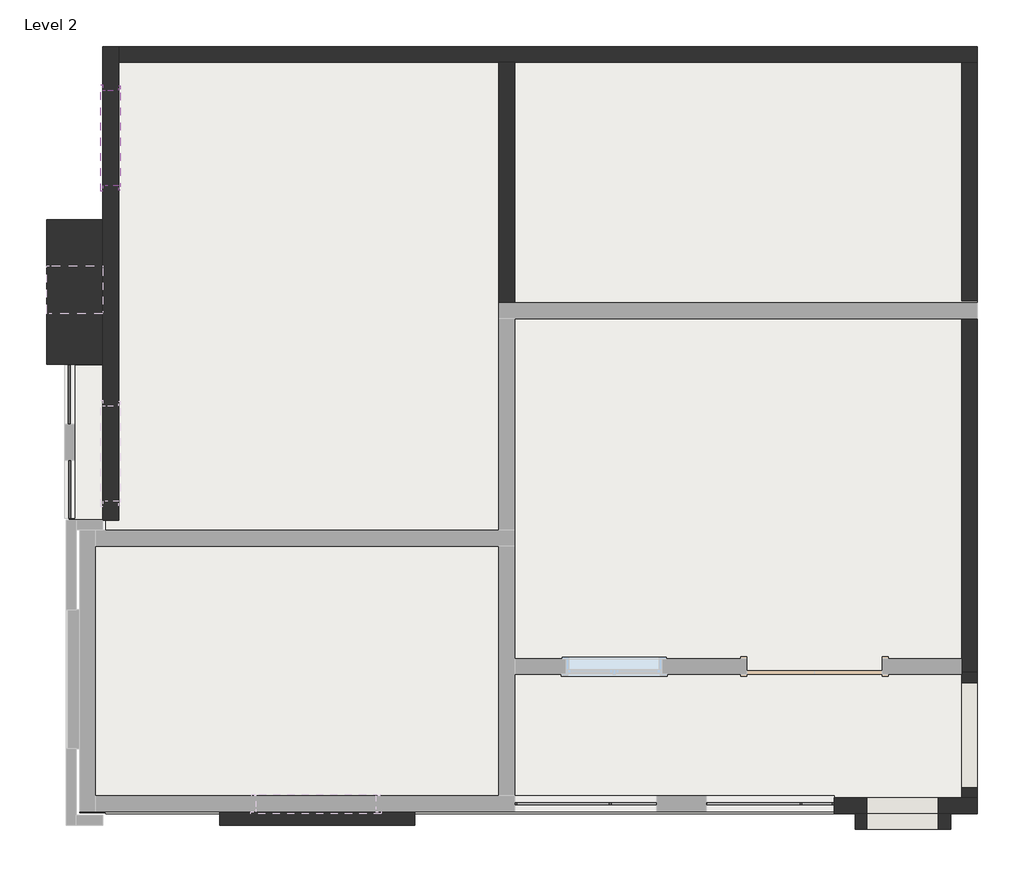
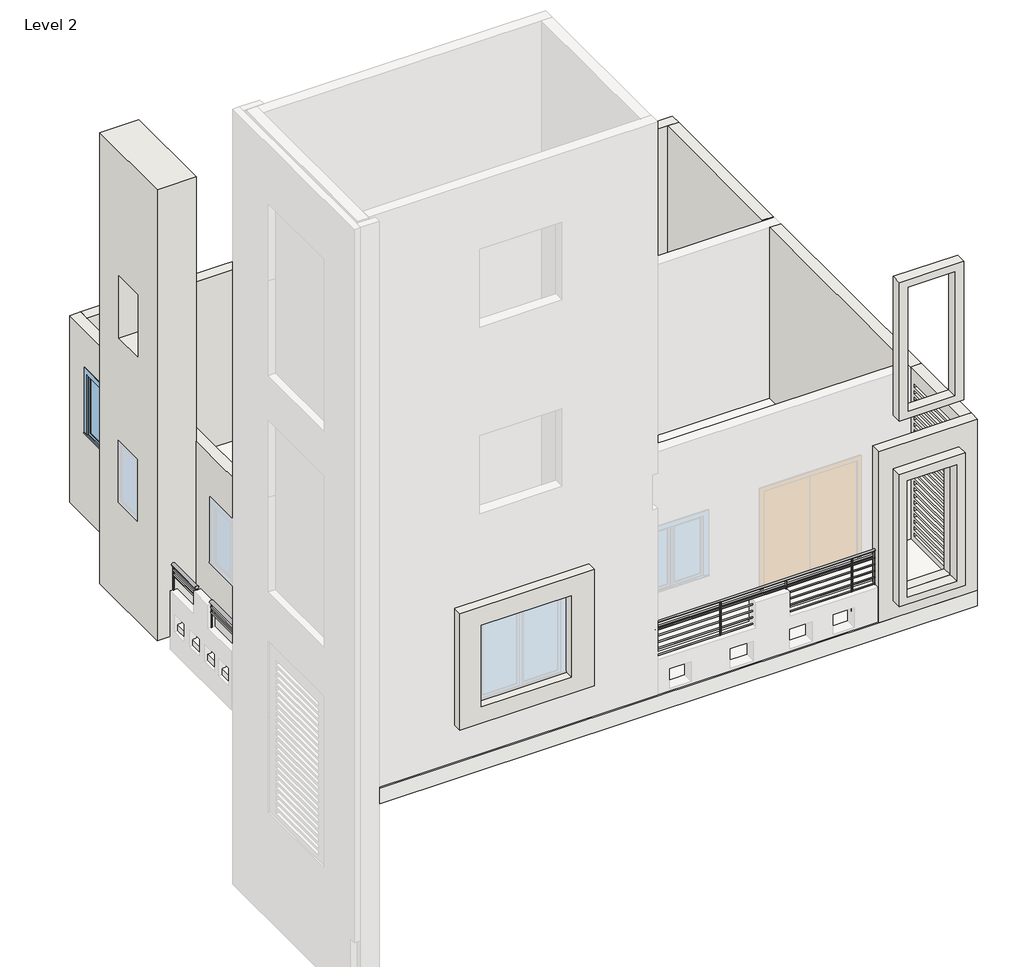
# One storey, part 2 of 2: 10 walls, 3 railings, 1 roof, 1 window.
"""IFC4 building model written with IfcOpenShell, lengths in millimetres."""

from ifc_helpers import new_model, si_unit, point, frame, frame_2d, origin, place, context, project, spatial, polyline, circle_curve, ellipse_curve, trimmed, segment, composite_curve, outline, extrude, faceted_brep, transform, mapped, element, save
from ifc_brep_helpers import plane_surface, extruded_surface, advanced_brep
from components import walls_1_walls_1_b1444295, walls_4_walls_4_8c60a96c, walls_5_walls_5_33b50d55, window_0862ab64

model = new_model("IFC4")

# Units and contexts
model_context = context("Model", 3, world=origin())
ifc_project = project(units=[si_unit("LENGTHUNIT", "METRE", prefix="MILLI")], contexts=[model_context])

# Site, building, storey
site = spatial("IfcSite", under=ifc_project)
building = spatial("IfcBuilding", under=site)
storey = spatial("IfcBuildingStorey", under=building, Name="Level 2", Elevation=3657.6)

# Railings
placement = place(None, origin())
element("IfcRailing", 1, ObjectType="Glass Panel - Bottom Fill", at=placement, inside=storey, context=model_context, shape_type="SolidModel", body=[
    advanced_brep(
    [(-10443.9247472, 7286.192958, 5059.6601563), (-10520.1247472, 7286.192958, 5059.6601563), (-10443.9247472, 6531.4144874, 5059.6601563), (-10520.1247472, 6531.4144874, 5059.6601563)],
    [
        (0, 1, ellipse_curve(frame((-10482.0247472, 7286.192958, 5059.6601563), z_axis=(0.0, 1.0, 0.0), x_axis=(-1.0, 0.0, 0.0)), 38.1, 28.575)),
        (1, 0, ellipse_curve(frame((-10482.0247472, 7286.192958, 5059.6601563), z_axis=(0.0, 1.0, 0.0), x_axis=(-1.0, 0.0, 0.0)), 38.1, 28.575)),
        (2, 3, ellipse_curve(frame((-10482.0247472, 6531.4144874, 5059.6601563), z_axis=(0.0, -1.0, 0.0), x_axis=(-1.0, 0.0, 0.0)), 38.1, 28.575)),
        (3, 2, ellipse_curve(frame((-10482.0247472, 6531.4144874, 5059.6601563), z_axis=(0.0, -1.0, 0.0), x_axis=(-1.0, 0.0, 0.0)), 38.1, 28.575)),
        (0, 2),
        (3, 1),
    ],
    [
        plane_surface(frame((-10482.0247472, 7286.192958, 5059.6601563), z_axis=(0.0, 1.0, 0.0), x_axis=(0.0, 0.0, -1.0))),
        plane_surface(frame((-10482.0247472, 6531.4144874, 5059.6601563), z_axis=(0.0, -1.0, 0.0), x_axis=(0.0, 0.0, -1.0))),
        extruded_surface(trimmed(ellipse_curve(frame((-10482.0247472, 6531.4144874, 5059.6601563), z_axis=(0.0, 1.0, 0.0), x_axis=(-1.0, 0.0, 0.0)), 38.1, 28.575), [point((-10443.9247472, 6531.4144874, 5059.6601563))], [point((-10520.1247472, 6531.4144874, 5059.6601563))], True, "CARTESIAN"), (0.0, 754.7784705999993, 0.0), 754.7784705999993),
        extruded_surface(trimmed(ellipse_curve(frame((-10482.0247472, 6531.4144874, 5059.6601563), z_axis=(0.0, 1.0, 0.0), x_axis=(-1.0, 0.0, 0.0)), 38.1, 28.575), [point((-10520.1247472, 6531.4144874, 5059.6601563))], [point((-10443.9247472, 6531.4144874, 5059.6601563))], True, "CARTESIAN"), (0.0, 754.7784705999993, 0.0), 754.7784705999993),
    ],
    [
        (0, [[1, 2]]),
        (1, [[3, 4]]),
        (2, [[-1, 5, -4, 6]]),
        (3, [[-2, -6, -3, -5]]),
    ],
),
    extrude(outline(polyline([(-10494.7247472, 7286.192958), (-10469.3247472, 7286.192958), (-10469.3247472, 6531.4144874), (-10494.7247472, 6531.4144874), (-10494.7247472, 7286.192958)])), frame((0.0, 0.0, 4945.3601562), z_axis=(0.0, 0.0, 1.0), x_axis=(1.0, 0.0, 0.0)), (0.0, 0.0, 1.0), 25.4),
    extrude(outline(polyline([(-10494.7247472, 7286.192958), (-10469.3247472, 7286.192958), (-10469.3247472, 6531.4144874), (-10494.7247472, 6531.4144874), (-10494.7247472, 7286.192958)])), frame((0.0, 0.0, 4843.7601563), z_axis=(0.0, 0.0, 1.0), x_axis=(1.0, 0.0, 0.0)), (0.0, 0.0, 1.0), 25.4),
    extrude(outline(polyline([(-10491.5497472, 6544.1144874), (-10472.4997472, 6544.1144874), (-10472.4997472, 6525.0644874), (-10491.5497472, 6525.0644874), (-10491.5497472, 6544.1144874)])), frame((0.0, 0.0, 4145.2601563), z_axis=(0.0, 0.0, 1.0), x_axis=(1.0, 0.0, 0.0)), (0.0, 0.0, 1.0), 885.6788223),
    extrude(outline(polyline([(-10491.5497472, 7292.542958), (-10472.4997472, 7292.542958), (-10472.4997472, 7273.492958), (-10491.5497472, 7273.492958), (-10491.5497472, 7292.542958)])), frame((0.0, 0.0, 4145.2601563), z_axis=(0.0, 0.0, 1.0), x_axis=(1.0, 0.0, 0.0)), (0.0, 0.0, 1.0), 885.6788223),
])
element("IfcRailing", 2, ObjectType="Glass Panel - Bottom Fill", at=placement, inside=storey, context=model_context, shape_type="SolidModel", body=[
    advanced_brep(
    [(-10437.5747472, 6074.2144874, 5059.6601563), (-10513.7747472, 6074.2144874, 5059.6601563), (-10437.5747472, 5330.392958, 5059.6601563), (-10513.7747472, 5330.392958, 5059.6601563)],
    [
        (0, 1, ellipse_curve(frame((-10475.6747472, 6074.2144874, 5059.6601563), z_axis=(0.0, 1.0, 0.0), x_axis=(-1.0, 0.0, 0.0)), 38.1, 28.575)),
        (1, 0, ellipse_curve(frame((-10475.6747472, 6074.2144874, 5059.6601563), z_axis=(0.0, 1.0, 0.0), x_axis=(-1.0, 0.0, 0.0)), 38.1, 28.575)),
        (2, 3, ellipse_curve(frame((-10475.6747472, 5330.392958, 5059.6601563), z_axis=(0.0, -1.0, 0.0), x_axis=(-1.0, 0.0, 0.0)), 38.1, 28.575)),
        (3, 2, ellipse_curve(frame((-10475.6747472, 5330.392958, 5059.6601563), z_axis=(0.0, -1.0, 0.0), x_axis=(-1.0, 0.0, 0.0)), 38.1, 28.575)),
        (0, 2),
        (3, 1),
    ],
    [
        plane_surface(frame((-10475.6747472, 6074.2144874, 5059.6601563), z_axis=(0.0, 1.0, 0.0), x_axis=(0.0, 0.0, -1.0))),
        plane_surface(frame((-10475.6747472, 5330.392958, 5059.6601563), z_axis=(0.0, -1.0, 0.0), x_axis=(0.0, 0.0, -1.0))),
        extruded_surface(trimmed(ellipse_curve(frame((-10475.6747472, 5330.392958, 5059.6601563), z_axis=(0.0, 1.0, 0.0), x_axis=(-1.0, 0.0, 0.0)), 38.1, 28.575), [point((-10437.5747472, 5330.392958, 5059.6601563))], [point((-10513.7747472, 5330.392958, 5059.6601563))], True, "CARTESIAN"), (0.0, 743.8215293999992, 0.0), 743.8215293999992),
        extruded_surface(trimmed(ellipse_curve(frame((-10475.6747472, 5330.392958, 5059.6601563), z_axis=(0.0, 1.0, 0.0), x_axis=(-1.0, 0.0, 0.0)), 38.1, 28.575), [point((-10513.7747472, 5330.392958, 5059.6601563))], [point((-10437.5747472, 5330.392958, 5059.6601563))], True, "CARTESIAN"), (0.0, 743.8215293999992, 0.0), 743.8215293999992),
    ],
    [
        (0, [[1, 2]]),
        (1, [[3, 4]]),
        (2, [[-1, 5, -4, 6]]),
        (3, [[-2, -6, -3, -5]]),
    ],
),
    extrude(outline(polyline([(-10488.3747472, 6074.2144874), (-10462.9747472, 6074.2144874), (-10462.9747472, 5330.392958), (-10488.3747472, 5330.392958), (-10488.3747472, 6074.2144874)])), frame((0.0, 0.0, 4945.3601562), z_axis=(0.0, 0.0, 1.0), x_axis=(1.0, 0.0, 0.0)), (0.0, 0.0, 1.0), 25.4),
    extrude(outline(polyline([(-10488.3747472, 6074.2144874), (-10462.9747472, 6074.2144874), (-10462.9747472, 5330.392958), (-10488.3747472, 5330.392958), (-10488.3747472, 6074.2144874)])), frame((0.0, 0.0, 4843.7601563), z_axis=(0.0, 0.0, 1.0), x_axis=(1.0, 0.0, 0.0)), (0.0, 0.0, 1.0), 25.4),
    extrude(outline(polyline([(-10485.1997472, 5343.092958), (-10466.1497472, 5343.092958), (-10466.1497472, 5324.042958), (-10485.1997472, 5324.042958), (-10485.1997472, 5343.092958)])), frame((0.0, 0.0, 4145.2601563), z_axis=(0.0, 0.0, 1.0), x_axis=(1.0, 0.0, 0.0)), (0.0, 0.0, 1.0), 885.6788223),
    extrude(outline(polyline([(-10485.1997472, 6080.5644874), (-10466.1497472, 6080.5644874), (-10466.1497472, 6061.5144874), (-10485.1997472, 6061.5144874), (-10485.1997472, 6080.5644874)])), frame((0.0, 0.0, 4145.2601563), z_axis=(0.0, 0.0, 1.0), x_axis=(1.0, 0.0, 0.0)), (0.0, 0.0, 1.0), 885.6788223),
])
element("IfcRailing", 3, ObjectType="Guardrail - Pipe", at=placement, inside=storey, context=model_context, shape_type="SweptSolid", body=[
    extrude(outline(composite_curve([segment(trimmed(circle_curve(frame_2d((1758.4484482, 5162.55)), 19.05), [point((1739.3984482, 5162.55))], [point((1777.4984482, 5162.55))], False, "CARTESIAN"), True, "CONTINUOUS"), segment(trimmed(circle_curve(frame_2d((1758.4484482, 5162.55)), 19.05), [point((1777.4984482, 5162.55))], [point((1739.3984482, 5162.55))], False, "CARTESIAN"), True, "CONTINUOUS")], self_intersect=False)), frame((-4789.9857575, 0.0, 0.0), z_axis=(1.0, 0.0, 0.0), x_axis=(0.0, 1.0, 0.0)), (0.0, 0.0, 1.0), 4083.7860103),
    extrude(outline(composite_curve([segment(trimmed(circle_curve(frame_2d((1682.2484482, 5314.95)), 19.05), [point((1663.1984482, 5314.95))], [point((1701.2984482, 5314.95))], False, "CARTESIAN"), True, "CONTINUOUS"), segment(trimmed(circle_curve(frame_2d((1682.2484482, 5314.95)), 19.05), [point((1701.2984482, 5314.95))], [point((1663.1984482, 5314.95))], False, "CARTESIAN"), True, "CONTINUOUS")], self_intersect=False)), frame((-4789.9857575, 0.0, 0.0), z_axis=(1.0, 0.0, 0.0), x_axis=(0.0, 1.0, 0.0)), (0.0, 0.0, 1.0), 4083.7860103),
    extrude(outline(composite_curve([segment(trimmed(circle_curve(frame_2d((1682.2484482, 5168.9)), 12.7), [point((1694.9484482, 5168.9))], [point((1669.5484482, 5168.9))], False, "CARTESIAN"), True, "CONTINUOUS"), segment(trimmed(circle_curve(frame_2d((1682.2484482, 5168.9)), 12.7), [point((1669.5484482, 5168.9))], [point((1694.9484482, 5168.9))], False, "CARTESIAN"), True, "CONTINUOUS")], self_intersect=False)), frame((-4789.9857575, 0.0, 0.0), z_axis=(1.0, 0.0, 0.0), x_axis=(0.0, 1.0, 0.0)), (0.0, 0.0, 1.0), 4083.7860103),
    extrude(outline(composite_curve([segment(trimmed(circle_curve(frame_2d((1682.2484482, 5041.9)), 12.7), [point((1694.9484482, 5041.9))], [point((1669.5484482, 5041.9))], False, "CARTESIAN"), True, "CONTINUOUS"), segment(trimmed(circle_curve(frame_2d((1682.2484482, 5041.9)), 12.7), [point((1669.5484482, 5041.9))], [point((1694.9484482, 5041.9))], False, "CARTESIAN"), True, "CONTINUOUS")], self_intersect=False)), frame((-4789.9857575, 0.0, 0.0), z_axis=(1.0, 0.0, 0.0), x_axis=(0.0, 1.0, 0.0)), (0.0, 0.0, 1.0), 4083.7860103),
    extrude(outline(composite_curve([segment(trimmed(circle_curve(frame_2d((1682.2484482, 4914.9)), 12.7), [point((1694.9484482, 4914.9))], [point((1669.5484482, 4914.9))], False, "CARTESIAN"), True, "CONTINUOUS"), segment(trimmed(circle_curve(frame_2d((1682.2484482, 4914.9)), 12.7), [point((1669.5484482, 4914.9))], [point((1694.9484482, 4914.9))], False, "CARTESIAN"), True, "CONTINUOUS")], self_intersect=False)), frame((-4789.9857575, 0.0, 0.0), z_axis=(1.0, 0.0, 0.0), x_axis=(0.0, 1.0, 0.0)), (0.0, 0.0, 1.0), 4083.7860103),
    extrude(outline(composite_curve([segment(trimmed(circle_curve(frame_2d((1682.2484482, 4787.9)), 12.7), [point((1694.9484482, 4787.9))], [point((1669.5484482, 4787.9))], False, "CARTESIAN"), True, "CONTINUOUS"), segment(trimmed(circle_curve(frame_2d((1682.2484482, 4787.9)), 12.7), [point((1669.5484482, 4787.9))], [point((1694.9484482, 4787.9))], False, "CARTESIAN"), True, "CONTINUOUS")], self_intersect=False)), frame((-4789.9857575, 0.0, 0.0), z_axis=(1.0, 0.0, 0.0), x_axis=(0.0, 1.0, 0.0)), (0.0, 0.0, 1.0), 4083.7860103),
    extrude(outline(composite_curve([segment(trimmed(circle_curve(frame_2d((1682.2484482, 4660.9)), 12.7), [point((1694.9484482, 4660.9))], [point((1669.5484482, 4660.9))], False, "CARTESIAN"), True, "CONTINUOUS"), segment(trimmed(circle_curve(frame_2d((1682.2484482, 4660.9)), 12.7), [point((1669.5484482, 4660.9))], [point((1694.9484482, 4660.9))], False, "CARTESIAN"), True, "CONTINUOUS")], self_intersect=False)), frame((-4789.9857575, 0.0, 0.0), z_axis=(1.0, 0.0, 0.0), x_axis=(0.0, 1.0, 0.0)), (0.0, 0.0, 1.0), 4083.7860103),
    extrude(outline(composite_curve([segment(trimmed(circle_curve(frame_2d((1682.2484482, 4533.9)), 12.7), [point((1694.9484482, 4533.9))], [point((1669.5484482, 4533.9))], False, "CARTESIAN"), True, "CONTINUOUS"), segment(trimmed(circle_curve(frame_2d((1682.2484482, 4533.9)), 12.7), [point((1669.5484482, 4533.9))], [point((1694.9484482, 4533.9))], False, "CARTESIAN"), True, "CONTINUOUS")], self_intersect=False)), frame((-4789.9857575, 0.0, 0.0), z_axis=(1.0, 0.0, 0.0), x_axis=(0.0, 1.0, 0.0)), (0.0, 0.0, 1.0), 4083.7860103),
    extrude(outline(composite_curve([segment(trimmed(circle_curve(frame_2d((1682.2484482, 4406.9)), 12.7), [point((1694.9484482, 4406.9))], [point((1669.5484482, 4406.9))], False, "CARTESIAN"), True, "CONTINUOUS"), segment(trimmed(circle_curve(frame_2d((1682.2484482, 4406.9)), 12.7), [point((1669.5484482, 4406.9))], [point((1694.9484482, 4406.9))], False, "CARTESIAN"), True, "CONTINUOUS")], self_intersect=False)), frame((-4789.9857575, 0.0, 0.0), z_axis=(1.0, 0.0, 0.0), x_axis=(0.0, 1.0, 0.0)), (0.0, 0.0, 1.0), 4083.7860103),
    extrude(outline(composite_curve([segment(trimmed(circle_curve(frame_2d((-1132.3857575, 1682.2484482)), 12.7), [point((-1132.3857575, 1694.9484482))], [point((-1132.3857575, 1669.5484482))], False, "CARTESIAN"), True, "CONTINUOUS"), segment(trimmed(circle_curve(frame_2d((-1132.3857575, 1682.2484482)), 12.7), [point((-1132.3857575, 1669.5484482))], [point((-1132.3857575, 1694.9484482))], False, "CARTESIAN"), True, "CONTINUOUS")], self_intersect=False)), frame((0.0, 0.0, 4267.2), z_axis=(0.0, 0.0, 1.0), x_axis=(1.0, 0.0, 0.0)), (0.0, 0.0, 1.0), 1028.7),
    extrude(outline(composite_curve([segment(trimmed(circle_curve(frame_2d((-2351.5857575, 1682.2484482)), 12.7), [point((-2351.5857575, 1694.9484482))], [point((-2351.5857575, 1669.5484482))], False, "CARTESIAN"), True, "CONTINUOUS"), segment(trimmed(circle_curve(frame_2d((-2351.5857575, 1682.2484482)), 12.7), [point((-2351.5857575, 1669.5484482))], [point((-2351.5857575, 1694.9484482))], False, "CARTESIAN"), True, "CONTINUOUS")], self_intersect=False)), frame((0.0, 0.0, 4267.2), z_axis=(0.0, 0.0, 1.0), x_axis=(1.0, 0.0, 0.0)), (0.0, 0.0, 1.0), 1028.7),
    extrude(outline(composite_curve([segment(trimmed(circle_curve(frame_2d((-3570.7857575, 1682.2484482)), 12.7), [point((-3570.7857575, 1694.9484482))], [point((-3570.7857575, 1669.5484482))], False, "CARTESIAN"), True, "CONTINUOUS"), segment(trimmed(circle_curve(frame_2d((-3570.7857575, 1682.2484482)), 12.7), [point((-3570.7857575, 1669.5484482))], [point((-3570.7857575, 1694.9484482))], False, "CARTESIAN"), True, "CONTINUOUS")], self_intersect=False)), frame((0.0, 0.0, 4267.2), z_axis=(0.0, 0.0, 1.0), x_axis=(1.0, 0.0, 0.0)), (0.0, 0.0, 1.0), 1028.7),
    extrude(outline(composite_curve([segment(trimmed(circle_curve(frame_2d((-718.8997472, 1682.2484482)), 12.7), [point((-718.8997472, 1694.9484482))], [point((-718.8997472, 1669.5484482))], False, "CARTESIAN"), True, "CONTINUOUS"), segment(trimmed(circle_curve(frame_2d((-718.8997472, 1682.2484482)), 12.7), [point((-718.8997472, 1669.5484482))], [point((-718.8997472, 1694.9484482))], False, "CARTESIAN"), True, "CONTINUOUS")], self_intersect=False)), frame((0.0, 0.0, 4267.2), z_axis=(0.0, 0.0, 1.0), x_axis=(1.0, 0.0, 0.0)), (0.0, 0.0, 1.0), 1028.7),
    extrude(outline(composite_curve([segment(trimmed(circle_curve(frame_2d((-4777.2857575, 1682.2484482)), 12.7), [point((-4777.2857575, 1694.9484482))], [point((-4777.2857575, 1669.5484482))], False, "CARTESIAN"), True, "CONTINUOUS"), segment(trimmed(circle_curve(frame_2d((-4777.2857575, 1682.2484482)), 12.7), [point((-4777.2857575, 1669.5484482))], [point((-4777.2857575, 1694.9484482))], False, "CARTESIAN"), True, "CONTINUOUS")], self_intersect=False)), frame((0.0, 0.0, 4267.2), z_axis=(0.0, 0.0, 1.0), x_axis=(1.0, 0.0, 0.0)), (0.0, 0.0, 1.0), 1028.7),
])

# Roof
element("IfcRoof", 4, ObjectType="Generic - 12\"", at=placement, inside=storey, context=model_context, shape_type="SweptSolid", body=[
    extrude(outline(polyline([(-10018.4747472, 11358.0609482), (1122.6002528, 11358.0609482), (1122.6002528, 1553.6609482), (-10019.8638097, 1553.6609482), (-10019.8638097, 1567.9484482), (-10352.5857575, 1567.9484482), (-10352.5857575, 5144.9959854), (-10018.4747472, 5144.9959854), (-10018.4747472, 5317.692958), (-10482.0247472, 5317.692958), (-10482.0247472, 7286.192958), (-10018.4747472, 7286.192958), (-10018.4747472, 11358.0609482)])), frame((0.0, 0.0, 3657.6), z_axis=(0.0, 0.0, 1.0), x_axis=(1.0, 0.0, 0.0)), (0.0, 0.0, 1.0), 304.8),
])

# Walls
element("IfcWall", 5, ObjectType="Generic - 8\"", at=placement, inside=storey, context=model_context, shape_type="Brep", body=[
    faceted_brep([(-9850.1997472, 5306.9209854, 3657.6), (-9850.1997472, 11154.8609482, 3657.6), (-9850.1997472, 11358.0609482, 3657.6), (-9850.1997472, 11358.0609482, 7315.2), (-9850.1997472, 11154.8609482, 7315.2), (-9850.1997472, 5306.9209854, 7315.2), (-9850.1997472, 6767.4209854, 6438.0362177), (-9850.1997472, 6767.4209854, 5218.8362177), (-9850.1997472, 5548.2209854, 5218.8362177), (-9850.1997472, 5548.2209854, 6438.0362177), (-9850.1997472, 10799.2609482, 6532.8486816), (-9850.1997472, 10799.2609482, 5313.6486816), (-9850.1997472, 9580.0609482, 5313.6486816), (-9850.1997472, 9580.0609482, 6532.8486816), (-10053.3997472, 5306.9209854, 3657.6), (-10053.3997472, 5306.9209854, 7315.2), (-10053.3997472, 11358.0609482, 7315.2), (-10053.3997472, 11358.0609482, 3657.6), (-10053.3997472, 6767.4209854, 6438.0362177), (-10053.3997472, 5548.2209854, 6438.0362177), (-10053.3997472, 5548.2209854, 5218.8362177), (-10053.3997472, 6767.4209854, 5218.8362177), (-10053.3997472, 10799.2609482, 6532.8486816), (-10053.3997472, 9580.0609482, 6532.8486816), (-10053.3997472, 9580.0609482, 5313.6486816), (-10053.3997472, 10799.2609482, 5313.6486816)], [[[0, 1, 2, 3, 4, 5], [6, 7, 8, 9], [10, 11, 12, 13]], [[14, 15, 16, 17], [18, 19, 20, 21], [22, 23, 24, 25]], [[2, 1, 0, 14, 17]], [[5, 4, 3, 16, 15]], [[0, 5, 15, 14]], [[3, 2, 17, 16]], [[7, 6, 18, 21]], [[8, 7, 21, 20]], [[9, 8, 20, 19]], [[6, 9, 19, 18]], [[11, 10, 22, 25]], [[12, 11, 25, 24]], [[13, 12, 24, 23]], [[10, 13, 23, 22]]]),
])
element("IfcWall", 6, ObjectType="Generic - 8\"", at=placement, inside=storey, context=model_context, shape_type="Brep", body=[
    faceted_brep([(-9850.1997472, 11154.8609482, 3657.6), (-4993.1857575, 11154.8609482, 3657.6), (-4789.9857575, 11154.8609482, 3657.6), (919.4002528, 11154.8609482, 3657.6), (1122.6002528, 11154.8609482, 3657.6), (1122.6002528, 11154.8609482, 7315.2), (919.4002528, 11154.8609482, 7315.2), (-4789.9857575, 11154.8609482, 7315.2), (-4993.1857575, 11154.8609482, 7315.2), (-9850.1997472, 11154.8609482, 7315.2), (-9850.1997472, 11358.0609482, 3657.6), (-9850.1997472, 11358.0609482, 7315.2), (1122.6002528, 11358.0609482, 7315.2), (1122.6002528, 11358.0609482, 3657.6)], [[[0, 1, 2, 3, 4, 5, 6, 7, 8, 9]], [[10, 11, 12, 13]], [[4, 3, 2, 1, 0, 10, 13]], [[9, 8, 7, 6, 5, 12, 11]], [[0, 9, 11, 10]], [[5, 4, 13, 12]]]),
])
element("IfcWall", 7, ObjectType="Generic - 8\"", at=placement, inside=storey, context=model_context, shape_type="SweptSolid", body=[
    extrude(outline(polyline([(919.4002528, 8106.8609482), (919.4002528, 11154.8609482), (1122.6002528, 11154.8609482), (1122.6002528, 8106.8609482), (919.4002528, 8106.8609482)])), frame((0.0, 0.0, 3657.6), z_axis=(0.0, 0.0, 1.0), x_axis=(1.0, 0.0, 0.0)), (0.0, 0.0, 1.0), 3657.6),
])
element("IfcWall", 8, ObjectType="Generic - 8\"", at=placement, inside=storey, context=model_context, shape_type="SweptSolid", body=[
    extrude(outline(polyline([(-4789.9857575, 11154.8609482), (-4789.9857575, 8083.0484482), (-4993.1857575, 8083.0484482), (-4993.1857575, 11154.8609482), (-4789.9857575, 11154.8609482)])), frame((0.0, 0.0, 3657.6), z_axis=(0.0, 0.0, 1.0), x_axis=(1.0, 0.0, 0.0)), (0.0, 0.0, 1.0), 3657.6),
])
element("IfcWall", 9, ObjectType="Generic - 8\"", at=placement, inside=storey, context=model_context, shape_type="Brep", body=[
    faceted_brep([(1122.6002528, 1756.8609482, 3961.5124256), (-706.1997472, 1756.8609482, 3961.5124256), (-706.1997472, 1756.8609482, 7315.2), (1122.6002528, 1756.8609482, 7315.2), (1122.6002528, 1756.8609482, 3962.4), (622.4491298, 1756.8609482, 6722.2388367), (-291.9508702, 1756.8609482, 6722.2388367), (-291.9508702, 1756.8609482, 4436.2388367), (622.4491298, 1756.8609482, 4436.2388367), (1122.6002528, 1553.6609482, 3961.5124256), (1122.6002528, 1553.6609482, 7315.2), (-706.1997472, 1553.6609482, 7315.2), (-706.1997472, 1553.6609482, 3961.5124256), (622.4491298, 1553.6609482, 6722.2388367), (622.4491298, 1553.6609482, 4436.2388367), (-291.9508702, 1553.6609482, 4436.2388367), (-291.9508702, 1553.6609482, 6722.2388367)], [[[0, 1, 2, 3, 4], [5, 6, 7, 8]], [[9, 10, 11, 12], [13, 14, 15, 16]], [[1, 0, 9, 12]], [[3, 2, 11, 10]], [[6, 5, 13, 16]], [[7, 6, 16, 15]], [[8, 7, 15, 14]], [[5, 8, 14, 13]], [[0, 4, 3, 10, 9]], [[1, 12, 11, 2]]]),
])
element("IfcWall", 10, ObjectType="Generic - 8\"", at=placement, inside=storey, context=model_context, shape_type="Brep", body=[
    faceted_brep([(1122.6002528, 3358.6484482, 3962.4), (1122.6002528, 3358.6484482, 7315.2), (1122.6002528, 1756.8609482, 7315.2), (1122.6002528, 1756.8609482, 3962.4), (1122.6002528, 3333.2484482, 3962.4), (1122.6002528, 3228.8895121, 7056.6542182), (1122.6002528, 3228.8895121, 6993.1542182), (1122.6002528, 1882.6895121, 6993.1542182), (1122.6002528, 1882.6895121, 7056.6542182), (1122.6002528, 3228.8895121, 6929.6542182), (1122.6002528, 3228.8895121, 6866.1542182), (1122.6002528, 1882.6895121, 6866.1542182), (1122.6002528, 1882.6895121, 6929.6542182), (1122.6002528, 3228.8895121, 6802.6542182), (1122.6002528, 3228.8895121, 6739.1542182), (1122.6002528, 1882.6895121, 6739.1542182), (1122.6002528, 1882.6895121, 6802.6542182), (1122.6002528, 3228.8895121, 6675.6542182), (1122.6002528, 3228.8895121, 6612.1542182), (1122.6002528, 1882.6895121, 6612.1542182), (1122.6002528, 1882.6895121, 6675.6542182), (1122.6002528, 3228.8895121, 6548.6542182), (1122.6002528, 3228.8895121, 6485.1542182), (1122.6002528, 1882.6895121, 6485.1542182), (1122.6002528, 1882.6895121, 6548.6542182), (1122.6002528, 3228.8895121, 6421.6542182), (1122.6002528, 3228.8895121, 6358.1542182), (1122.6002528, 1882.6895121, 6358.1542182), (1122.6002528, 1882.6895121, 6421.6542182), (1122.6002528, 3228.8895121, 6294.6542182), (1122.6002528, 3228.8895121, 6231.1542182), (1122.6002528, 1882.6895121, 6231.1542182), (1122.6002528, 1882.6895121, 6294.6542182), (1122.6002528, 3228.8895121, 6167.6542182), (1122.6002528, 3228.8895121, 6104.1542182), (1122.6002528, 1882.6895121, 6104.1542182), (1122.6002528, 1882.6895121, 6167.6542182), (1122.6002528, 3228.8895121, 6040.6542182), (1122.6002528, 3228.8895121, 5977.1542182), (1122.6002528, 1882.6895121, 5977.1542182), (1122.6002528, 1882.6895121, 6040.6542182), (1122.6002528, 3228.8895121, 5913.6542182), (1122.6002528, 3228.8895121, 5850.1542182), (1122.6002528, 1882.6895121, 5850.1542182), (1122.6002528, 1882.6895121, 5913.6542182), (1122.6002528, 3228.8895121, 5786.6542182), (1122.6002528, 3228.8895121, 5723.1542182), (1122.6002528, 1882.6895121, 5723.1542182), (1122.6002528, 1882.6895121, 5786.6542182), (1122.6002528, 3228.8895121, 5659.6542182), (1122.6002528, 3228.8895121, 5596.1542182), (1122.6002528, 1882.6895121, 5596.1542182), (1122.6002528, 1882.6895121, 5659.6542182), (1122.6002528, 3228.8895121, 5532.6542182), (1122.6002528, 3228.8895121, 5469.1542182), (1122.6002528, 1882.6895121, 5469.1542182), (1122.6002528, 1882.6895121, 5532.6542182), (1122.6002528, 3228.8895121, 5405.6542182), (1122.6002528, 3228.8895121, 5342.1542182), (1122.6002528, 1882.6895121, 5342.1542182), (1122.6002528, 1882.6895121, 5405.6542182), (1122.6002528, 3228.8895121, 5278.6542182), (1122.6002528, 3228.8895121, 5215.1542182), (1122.6002528, 1882.6895121, 5215.1542182), (1122.6002528, 1882.6895121, 5278.6542182), (1122.6002528, 3228.8895121, 5151.6542182), (1122.6002528, 3228.8895121, 5088.1542182), (1122.6002528, 1882.6895121, 5088.1542182), (1122.6002528, 1882.6895121, 5151.6542182), (1122.6002528, 3228.8895121, 5024.6542182), (1122.6002528, 3228.8895121, 4961.1542182), (1122.6002528, 1882.6895121, 4961.1542182), (1122.6002528, 1882.6895121, 5024.6542182), (1122.6002528, 3228.8895121, 4897.6542182), (1122.6002528, 3228.8895121, 4834.1542182), (1122.6002528, 1882.6895121, 4834.1542182), (1122.6002528, 1882.6895121, 4897.6542182), (1122.6002528, 3228.8895121, 4770.6542182), (1122.6002528, 3228.8895121, 4707.1542182), (1122.6002528, 1882.6895121, 4707.1542182), (1122.6002528, 1882.6895121, 4770.6542182), (1122.6002528, 3228.8895121, 4643.6542182), (1122.6002528, 3228.8895121, 4580.1542182), (1122.6002528, 1882.6895121, 4580.1542182), (1122.6002528, 1882.6895121, 4643.6542182), (1122.6002528, 3228.8895121, 4516.6542182), (1122.6002528, 3228.8895121, 4453.1542182), (1122.6002528, 1882.6895121, 4453.1542182), (1122.6002528, 1882.6895121, 4516.6542182), (1122.6002528, 3228.8895121, 4389.6542182), (1122.6002528, 3228.8895121, 4326.1542182), (1122.6002528, 1882.6895121, 4326.1542182), (1122.6002528, 1882.6895121, 4389.6542182), (1122.6002528, 3228.8895121, 4262.6542182), (1122.6002528, 3228.8895121, 4199.1542182), (1122.6002528, 1882.6895121, 4199.1542182), (1122.6002528, 1882.6895121, 4262.6542182), (1122.6002528, 3228.8895121, 4135.6542182), (1122.6002528, 3228.8895121, 4072.1542182), (1122.6002528, 1882.6895121, 4072.1542182), (1122.6002528, 1882.6895121, 4135.6542182), (919.4002528, 3358.6484482, 3962.4), (919.4002528, 3333.2484482, 3962.4), (919.4002528, 1756.8609482, 3962.4), (919.4002528, 1756.8609482, 7315.2), (919.4002528, 3333.2484482, 7315.2), (919.4002528, 3358.6484482, 7315.2), (919.4002528, 3228.8895121, 7056.6542182), (919.4002528, 1882.6895121, 7056.6542182), (919.4002528, 1882.6895121, 6993.1542182), (919.4002528, 3228.8895121, 6993.1542182), (919.4002528, 3228.8895121, 6929.6542182), (919.4002528, 1882.6895121, 6929.6542182), (919.4002528, 1882.6895121, 6866.1542182), (919.4002528, 3228.8895121, 6866.1542182), (919.4002528, 3228.8895121, 6802.6542182), (919.4002528, 1882.6895121, 6802.6542182), (919.4002528, 1882.6895121, 6739.1542182), (919.4002528, 3228.8895121, 6739.1542182), (919.4002528, 3228.8895121, 6675.6542182), (919.4002528, 1882.6895121, 6675.6542182), (919.4002528, 1882.6895121, 6612.1542182), (919.4002528, 3228.8895121, 6612.1542182), (919.4002528, 3228.8895121, 6548.6542182), (919.4002528, 1882.6895121, 6548.6542182), (919.4002528, 1882.6895121, 6485.1542182), (919.4002528, 3228.8895121, 6485.1542182), (919.4002528, 3228.8895121, 6421.6542182), (919.4002528, 1882.6895121, 6421.6542182), (919.4002528, 1882.6895121, 6358.1542182), (919.4002528, 3228.8895121, 6358.1542182), (919.4002528, 3228.8895121, 6294.6542182), (919.4002528, 1882.6895121, 6294.6542182), (919.4002528, 1882.6895121, 6231.1542182), (919.4002528, 3228.8895121, 6231.1542182), (919.4002528, 3228.8895121, 6167.6542182), (919.4002528, 1882.6895121, 6167.6542182), (919.4002528, 1882.6895121, 6104.1542182), (919.4002528, 3228.8895121, 6104.1542182), (919.4002528, 3228.8895121, 6040.6542182), (919.4002528, 1882.6895121, 6040.6542182), (919.4002528, 1882.6895121, 5977.1542182), (919.4002528, 3228.8895121, 5977.1542182), (919.4002528, 3228.8895121, 5913.6542182), (919.4002528, 1882.6895121, 5913.6542182), (919.4002528, 1882.6895121, 5850.1542182), (919.4002528, 3228.8895121, 5850.1542182), (919.4002528, 3228.8895121, 5786.6542182), (919.4002528, 1882.6895121, 5786.6542182), (919.4002528, 1882.6895121, 5723.1542182), (919.4002528, 3228.8895121, 5723.1542182), (919.4002528, 3228.8895121, 5659.6542182), (919.4002528, 1882.6895121, 5659.6542182), (919.4002528, 1882.6895121, 5596.1542182), (919.4002528, 3228.8895121, 5596.1542182), (919.4002528, 3228.8895121, 5532.6542182), (919.4002528, 1882.6895121, 5532.6542182), (919.4002528, 1882.6895121, 5469.1542182), (919.4002528, 3228.8895121, 5469.1542182), (919.4002528, 3228.8895121, 5405.6542182), (919.4002528, 1882.6895121, 5405.6542182), (919.4002528, 1882.6895121, 5342.1542182), (919.4002528, 3228.8895121, 5342.1542182), (919.4002528, 3228.8895121, 5278.6542182), (919.4002528, 1882.6895121, 5278.6542182), (919.4002528, 1882.6895121, 5215.1542182), (919.4002528, 3228.8895121, 5215.1542182), (919.4002528, 3228.8895121, 5151.6542182), (919.4002528, 1882.6895121, 5151.6542182), (919.4002528, 1882.6895121, 5088.1542182), (919.4002528, 3228.8895121, 5088.1542182), (919.4002528, 3228.8895121, 5024.6542182), (919.4002528, 1882.6895121, 5024.6542182), (919.4002528, 1882.6895121, 4961.1542182), (919.4002528, 3228.8895121, 4961.1542182), (919.4002528, 3228.8895121, 4897.6542182), (919.4002528, 1882.6895121, 4897.6542182), (919.4002528, 1882.6895121, 4834.1542182), (919.4002528, 3228.8895121, 4834.1542182), (919.4002528, 3228.8895121, 4770.6542182), (919.4002528, 1882.6895121, 4770.6542182), (919.4002528, 1882.6895121, 4707.1542182), (919.4002528, 3228.8895121, 4707.1542182), (919.4002528, 3228.8895121, 4643.6542182), (919.4002528, 1882.6895121, 4643.6542182), (919.4002528, 1882.6895121, 4580.1542182), (919.4002528, 3228.8895121, 4580.1542182), (919.4002528, 3228.8895121, 4516.6542182), (919.4002528, 1882.6895121, 4516.6542182), (919.4002528, 1882.6895121, 4453.1542182), (919.4002528, 3228.8895121, 4453.1542182), (919.4002528, 3228.8895121, 4389.6542182), (919.4002528, 1882.6895121, 4389.6542182), (919.4002528, 1882.6895121, 4326.1542182), (919.4002528, 3228.8895121, 4326.1542182), (919.4002528, 3228.8895121, 4262.6542182), (919.4002528, 1882.6895121, 4262.6542182), (919.4002528, 1882.6895121, 4199.1542182), (919.4002528, 3228.8895121, 4199.1542182), (919.4002528, 3228.8895121, 4135.6542182), (919.4002528, 1882.6895121, 4135.6542182), (919.4002528, 1882.6895121, 4072.1542182), (919.4002528, 3228.8895121, 4072.1542182)], [[[0, 1, 2, 3, 4], [5, 6, 7, 8], [9, 10, 11, 12], [13, 14, 15, 16], [17, 18, 19, 20], [21, 22, 23, 24], [25, 26, 27, 28], [29, 30, 31, 32], [33, 34, 35, 36], [37, 38, 39, 40], [41, 42, 43, 44], [45, 46, 47, 48], [49, 50, 51, 52], [53, 54, 55, 56], [57, 58, 59, 60], [61, 62, 63, 64], [65, 66, 67, 68], [69, 70, 71, 72], [73, 74, 75, 76], [77, 78, 79, 80], [81, 82, 83, 84], [85, 86, 87, 88], [89, 90, 91, 92], [93, 94, 95, 96], [97, 98, 99, 100]], [[101, 102, 103, 104, 105, 106], [107, 108, 109, 110], [111, 112, 113, 114], [115, 116, 117, 118], [119, 120, 121, 122], [123, 124, 125, 126], [127, 128, 129, 130], [131, 132, 133, 134], [135, 136, 137, 138], [139, 140, 141, 142], [143, 144, 145, 146], [147, 148, 149, 150], [151, 152, 153, 154], [155, 156, 157, 158], [159, 160, 161, 162], [163, 164, 165, 166], [167, 168, 169, 170], [171, 172, 173, 174], [175, 176, 177, 178], [179, 180, 181, 182], [183, 184, 185, 186], [187, 188, 189, 190], [191, 192, 193, 194], [195, 196, 197, 198], [199, 200, 201, 202]], [[0, 4, 3, 103, 102, 101]], [[2, 1, 106, 105, 104]], [[1, 0, 101, 106]], [[3, 2, 104, 103]], [[6, 5, 107, 110]], [[7, 6, 110, 109]], [[8, 7, 109, 108]], [[5, 8, 108, 107]], [[10, 9, 111, 114]], [[11, 10, 114, 113]], [[12, 11, 113, 112]], [[9, 12, 112, 111]], [[14, 13, 115, 118]], [[15, 14, 118, 117]], [[16, 15, 117, 116]], [[13, 16, 116, 115]], [[18, 17, 119, 122]], [[19, 18, 122, 121]], [[20, 19, 121, 120]], [[17, 20, 120, 119]], [[22, 21, 123, 126]], [[23, 22, 126, 125]], [[24, 23, 125, 124]], [[21, 24, 124, 123]], [[26, 25, 127, 130]], [[27, 26, 130, 129]], [[28, 27, 129, 128]], [[25, 28, 128, 127]], [[30, 29, 131, 134]], [[31, 30, 134, 133]], [[32, 31, 133, 132]], [[29, 32, 132, 131]], [[34, 33, 135, 138]], [[35, 34, 138, 137]], [[36, 35, 137, 136]], [[33, 36, 136, 135]], [[38, 37, 139, 142]], [[39, 38, 142, 141]], [[40, 39, 141, 140]], [[37, 40, 140, 139]], [[42, 41, 143, 146]], [[43, 42, 146, 145]], [[44, 43, 145, 144]], [[41, 44, 144, 143]], [[46, 45, 147, 150]], [[47, 46, 150, 149]], [[48, 47, 149, 148]], [[45, 48, 148, 147]], [[50, 49, 151, 154]], [[51, 50, 154, 153]], [[52, 51, 153, 152]], [[49, 52, 152, 151]], [[54, 53, 155, 158]], [[55, 54, 158, 157]], [[56, 55, 157, 156]], [[53, 56, 156, 155]], [[58, 57, 159, 162]], [[59, 58, 162, 161]], [[60, 59, 161, 160]], [[57, 60, 160, 159]], [[62, 61, 163, 166]], [[63, 62, 166, 165]], [[64, 63, 165, 164]], [[61, 64, 164, 163]], [[66, 65, 167, 170]], [[67, 66, 170, 169]], [[68, 67, 169, 168]], [[65, 68, 168, 167]], [[70, 69, 171, 174]], [[71, 70, 174, 173]], [[72, 71, 173, 172]], [[69, 72, 172, 171]], [[74, 73, 175, 178]], [[75, 74, 178, 177]], [[76, 75, 177, 176]], [[73, 76, 176, 175]], [[78, 77, 179, 182]], [[79, 78, 182, 181]], [[80, 79, 181, 180]], [[77, 80, 180, 179]], [[82, 81, 183, 186]], [[83, 82, 186, 185]], [[84, 83, 185, 184]], [[81, 84, 184, 183]], [[86, 85, 187, 190]], [[87, 86, 190, 189]], [[88, 87, 189, 188]], [[85, 88, 188, 187]], [[90, 89, 191, 194]], [[91, 90, 194, 193]], [[92, 91, 193, 192]], [[89, 92, 192, 191]], [[94, 93, 195, 198]], [[95, 94, 198, 197]], [[96, 95, 197, 196]], [[93, 96, 196, 195]], [[98, 97, 199, 202]], [[99, 98, 202, 201]], [[100, 99, 201, 200]], [[97, 100, 200, 199]]]),
])
element("IfcWall", 11, ObjectType="Generic - 8\"", at=placement, inside=storey, context=model_context, shape_type="Brep", body=[
    faceted_brep([(1122.6002528, 3333.2484482, 3657.6), (1122.6002528, 7879.8484482, 3657.6), (1122.6002528, 7879.8484482, 7315.2), (1122.6002528, 3358.6484482, 7315.2), (1122.6002528, 3358.6484482, 3962.4), (1122.6002528, 3333.2484482, 3962.4), (919.4002528, 3333.2484482, 3657.6), (919.4002528, 3333.2484482, 3962.4), (919.4002528, 3358.6484482, 3962.4), (919.4002528, 3358.6484482, 7315.2), (919.4002528, 3536.4484482, 7315.2), (919.4002528, 7879.8484482, 7315.2), (919.4002528, 7879.8484482, 3657.6), (919.4002528, 3536.4484482, 3657.6)], [[[0, 1, 2, 3, 4, 5]], [[6, 7, 8, 9, 10, 11, 12, 13]], [[1, 0, 6, 13, 12]], [[3, 2, 11, 10, 9]], [[2, 1, 12, 11]], [[4, 8, 7, 5]], [[3, 9, 8, 4]], [[0, 5, 7, 6]]]),
])
walls_1_walls_1_shape = walls_1_walls_1_b1444295(model_context)
element("IfcWall", 12, ObjectType="Walls 1 : Walls 1", at=placement, inside=storey, context=model_context, shape_type="MappedRepresentation", body=[
    mapped(walls_1_walls_1_shape, transform((0.0, 0.0, 0.0), x_axis=(1.0, 0.0, 0.0), y_axis=(0.0, 1.0, 0.0), z_axis=(0.0, 0.0, 1.0))),
])
walls_4_walls_4_shape = walls_4_walls_4_8c60a96c(model_context)
element("IfcWall", 13, ObjectType="Walls 4 : Walls 4", at=placement, inside=storey, context=model_context, shape_type="MappedRepresentation", body=[
    mapped(walls_4_walls_4_shape, transform((0.0, 0.0, 0.0), x_axis=(1.0, 0.0, 0.0), y_axis=(0.0, 1.0, 0.0), z_axis=(0.0, 0.0, 1.0))),
])
walls_5_walls_5_shape = walls_5_walls_5_33b50d55(model_context)
element("IfcWall", 14, ObjectType="Walls 5 : Walls 5", at=placement, inside=storey, context=model_context, shape_type="MappedRepresentation", body=[
    mapped(walls_5_walls_5_shape, transform((0.0, 0.0, 0.0), x_axis=(1.0, 0.0, 0.0), y_axis=(0.0, 1.0, 0.0), z_axis=(0.0, 0.0, 1.0))),
])

# Window
window_shape = window_0862ab64(model_context)
element("IfcWindow", 15, ObjectType="Casement Dbl with Trim : 48\" x 48\"", at=placement, inside=storey, context=model_context, shape_type="MappedRepresentation", body=[
    mapped(window_shape, transform((-9932.7497472, 10189.6609482, 4399.2486816), x_axis=(0.0, 1.0, 0.0), y_axis=(-1.0, 0.0, 0.0), z_axis=(0.0, 0.0, 1.0))),
])

save(model, "model.ifc")

# Revit data of these elements
# Type "Glass Panel - Bottom Fill"
#   Assembly Code = "C2010400"
#   built-in parameter 1008612 = 0.0416667 (stored number, unit not read)
#   built-in parameter 1008611 = 0.0416667 (stored number, unit not read)
#   built-in parameter 1008609 = 0.333333 (stored number, unit not read)
#   built-in parameter 1008604 = 0.166667 (stored number, unit not read)
#   built-in parameter 1008603 = 0.166667 (stored number, unit not read)
#   Railing Height = 3' - 0"
#   built-in parameter 1008630 = 2
#   built-in parameter 1008610 = 2
#   built-in parameter 1008618 = Baluster - Square : 3/4"
# Type "Guardrail - Pipe"
#   Assembly Code = "C2010400"
#   built-in parameter 1008612 = 0.0416667 (stored number, unit not read)
#   built-in parameter 1008611 = 0.0833333 (stored number, unit not read)
#   built-in parameter 1008609 = 4 (stored number, unit not read)
#   built-in parameter 1008604 = 0.166667 (stored number, unit not read)
#   built-in parameter 1008603 = 0.166667 (stored number, unit not read)
#   Railing Height = 3' - 6"
#   built-in parameter 1008630 = 2
#   built-in parameter 1008610 = 1
#   built-in parameter 1008605 = 1
#   built-in parameter 1008618 = Baluster - Round : 1"
# Type "Generic - 12\""
#   Assembly Code = "B1020"
#   Layers, outside or top first: 1' - 0" no material (function 1)
# Type "Generic - 8\""
#   Assembly Code = "B2010"
#   Layers, outside or top first: 0' - 8" no material (function 1)
# Type "Casement Dbl with Trim : 48\" x 48\""
#   Type Mark = "13"
#   Construction Type Id = "GSP4R"
#   Assembly Code = "B2020100"
#   Analytic Construction = "1/8 in Pilkington single glazing"
#   Visual Light Transmittance = 0.9
#   Thermal Resistance (R) = 1.53941 (h·ft²·°F)/BTU
#   Solar Heat Gain Coefficient = 0.78
#   Heat Transfer Coefficient (U) = 0.6496 BTU/(h·ft²·°F)
#   Height = 4' - 0"
#   Default Sill Height = 3' - 0"
#   Trim Projection - Ext. = 0' - 0 1/2"
#   Trim Projection - Int. = 0' - 0 3/4"
#   Trim Width - Exterior = 0' - 3 1/2"
#   Trim Width - Interior = 0' - 3 1/2"
#   Width = 4' - 0"
#   Window Inset = 0' - 0 3/4"
#   Define Thermal Properties by = 1
#   Glass Pane Material = Glass
#   Sash Material = Sash
#   Trim Exterior Material = Trim
#   Trim Interior Material = Trim
#   Wall Closure = (empty or 0)
# Elements 1, 2 (IfcRailing, "Glass Panel - Bottom Fill")
#   built-in parameter 1008621 = 1.59993 (stored number, unit not read)
#   Phase Created = New Construction
# Element 3 (IfcRailing, "Guardrail - Pipe")
#   built-in parameter 1008621 = 2 (stored number, unit not read)
#   Phase Created = New Construction
# Element 4 (IfcRoof, "Generic - 12\"")
#   built-in parameter 1001705 = 13 (stored number, unit not read)
#   built-in parameter 1001710 = 33615
#   Phase Created = New Construction
#   Materials on its faces: "Default Roof"
# Elements 5, 6, 7, 8, 11 (IfcWall, "Generic - 8\"")
#   Top Offset = 0' - 0"
#   Base Offset = 0' - 0"
#   Unconnected Height = 12' - 0"
#   wall height = 12' - 0"
#   Phase Created = New Construction
#   Base Constraint = Level 2
#   Materials on its faces: "Default Wall"
# Element 9 (IfcWall, "Generic - 8\"")
#   built-in parameter 1001111 = 0' - 11.96506"
#   Top Offset = 0' - 0"
#   Base Offset = 0' - 11.96506"
#   Unconnected Height = 11' - 0.03494"
#   wall height = 11' - 0.03494"
#   Phase Created = New Construction
#   Base Constraint = Level 2
#   Materials on its faces: "Default Wall"
# Element 10 (IfcWall, "Generic - 8\"")
#   built-in parameter 1001111 = 1' - 0"
#   Top Offset = 0' - 0"
#   Base Offset = 1' - 0"
#   Unconnected Height = 11' - 0"
#   wall height = 11' - 0"
#   Phase Created = New Construction
#   Base Constraint = Level 2
#   Materials on its faces: "Default Wall"
# Element 12 (IfcWall, "Walls 1 : Walls 1")
#   Phase Created = New Construction
#   Materials on its faces: "Default Wall"
# Element 13 (IfcWall, "Walls 4 : Walls 4")
#   Phase Created = New Construction
#   Materials on its faces: "Default Wall"
# Element 14 (IfcWall, "Walls 5 : Walls 5")
#   Phase Created = New Construction
#   Materials on its faces: "Default Wall"
# Element 15 (IfcWindow, "Casement Dbl with Trim : 48\" x 48\"")
#   Mark = "11"
#   Phase Created = New Construction
#   Materials on its faces: "Sash", "Trim", "Glass"
# Materials
#   "Glass": class "Glass", colour RGB 0 128 192, transparency 0.75, Description = "Soda Lime Glass", Cost = 0
#   "Sash": class "Wood", colour RGB 224 178 126, transparency 0
#   "Trim": class "Wood", colour RGB 224 178 126, transparency 0
#   "Default Roof": colour RGB 88 101 114, transparency 0
#   "Default Wall": colour RGB 128 128 128, transparency 0
